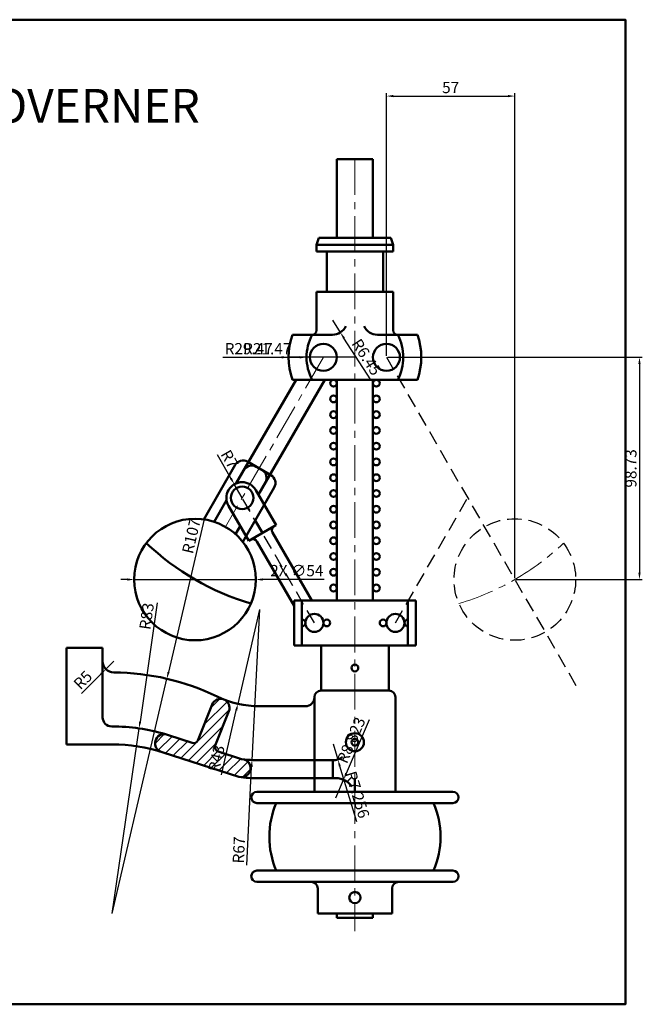
# Model space of a CAD drawing. Units: millimetres. Extents: x 98 to 674, y 38 to 476.
# Tile 7 of 7: x 398 to 674, y 38 to 476. Entities that reach past the tile are written whole.
import ezdxf

# ---------------------------------------------------------------- set-up
doc = ezdxf.new("R2010")
doc.units = ezdxf.units.MM
doc.header["$LTSCALE"] = 0.5
doc.linetypes.add('CENTER', pattern=[50.8, 31.75, -6.35, 6.35, -6.35])
doc.linetypes.add('DASHED', pattern=[19.05, 12.7, -6.35])
for name, color, linetype, lineweight in [('M-CNTR', 1, 'CENTER', 18), ('M-DIMS', 2, 'Continuous', 25), ('M-HATC', 8, 'Continuous', 18), ('M-OUTL', 7, 'Continuous', 50), ('M-PHAN', 6, 'DASHED', 25), ('M-TEXT', 3, 'Continuous', 25), ('M-TTLB', 7, 'Continuous', 50)]:
    doc.layers.add(name, color=color, linetype=linetype, lineweight=lineweight)
doc.styles.get("Standard").update_dxf_attribs({"font": 'arial.ttf'})
doc.dimstyles.new('ISO-25', dxfattribs={"dimtxt": 5, "dimasz": 3, "dimexe": 1.25, "dimexo": 0.625, "dimtad": 1, "dimtxsty": 'Standard', "dimcen": 2.5, "dimadec": 0, "dimazin": 0, "dimtfac": 1, "dimtmove": 0, "dimatfit": 3, "dimfxl": 1, "dimarcsym": 0})

# ---------------------------------------------------------------- blocks, each defined once
blk = doc.blocks.new('BALL')
blk.add_circle((27, 27), 27)
blk.add_arc((84, 125.73), 114, 226.398, 253.602)
blk = doc.blocks.new('*D69')
at = {"layer": 'Defpoints', "color": 0, "ltscale": 0.5, "transparency": 16777216}
for p in [(560.64, 325.69), (617.64, 226.96), (672.98, 226.96)]:
    blk.add_point(p, dxfattribs=at)
at = {"layer": 'M-DIMS', "color": 0, "lineweight": -2, "ltscale": 0.5, "transparency": 16777216}
for p, q in [((561.27, 325.69), (674.23, 325.69)), ((672.98, 322.69), (672.98, 229.96)), ((618.27, 226.96), (674.23, 226.96))]:
    blk.add_line(p, q, dxfattribs=at)
at = {"layer": 'M-DIMS', "color": 0, "ltscale": 0.5, "transparency": 16777216}
for points in [[(672.48, 322.69), (673.48, 322.69), (672.98, 325.69)], [(672.48, 229.96), (673.48, 229.96), (672.98, 226.96)]]:
    blk.add_solid(points, dxfattribs=at)
at = {"layer": 'M-DIMS', "color": 0, "ltscale": 0.5, "transparency": 16777216, "insert": (669.8, 276.32), "char_height": 5, "attachment_point": 5, "rotation": 90}
blk.add_mtext('98.73', dxfattribs=at)
blk = doc.blocks.new('*D70')
at = {"layer": 'Defpoints', "color": 0, "ltscale": 0.5, "transparency": 16777216}
for p in [(617.64, 441.69), (560.64, 325.69), (617.64, 226.96)]:
    blk.add_point(p, dxfattribs=at)
at = {"layer": 'M-DIMS', "color": 0, "lineweight": -2, "ltscale": 0.5, "transparency": 16777216}
for p, q in [((560.64, 326.31), (560.64, 442.94)), ((617.64, 227.58), (617.64, 442.94)), ((563.64, 441.69), (614.64, 441.69))]:
    blk.add_line(p, q, dxfattribs=at)
at = {"layer": 'M-DIMS', "color": 0, "ltscale": 0.5, "transparency": 16777216}
for points in [[(563.64, 442.19), (563.64, 441.19), (560.64, 441.69)], [(614.64, 442.19), (614.64, 441.19), (617.64, 441.69)]]:
    blk.add_solid(points, dxfattribs=at)
at = {"layer": 'M-DIMS', "color": 0, "ltscale": 0.5, "transparency": 16777216, "insert": (589.14, 444.85), "char_height": 5, "attachment_point": 5}
blk.add_mtext('57', dxfattribs=at)
blk = doc.blocks.new('*D75')
at = {"layer": 'Defpoints', "color": 0, "ltscale": 0.5, "transparency": 16777216}
for p in [(439.64, 190.68), (436.09, 187.16)]:
    blk.add_point(p, dxfattribs=at)
at = {"layer": 'M-DIMS', "color": 0, "lineweight": -2, "ltscale": 0.5, "transparency": 16777216}
for p, q in [((439.64, 190.68), (436.09, 187.16)), ((425.2, 176.34), (433.96, 185.04))]:
    blk.add_line(p, q, dxfattribs=at)
at = {"layer": 'M-DIMS', "color": 0, "ltscale": 0.5, "transparency": 16777216}
blk.add_solid([(433.61, 185.4), (434.32, 184.69), (436.09, 187.16)], dxfattribs=at)
at = {"layer": 'M-DIMS', "color": 0, "ltscale": 0.5, "transparency": 16777216, "insert": (426.29, 181.88), "char_height": 5, "attachment_point": 5, "rotation": 44.812}
blk.add_mtext('R5', dxfattribs=at)
blk = doc.blocks.new('*D79')
at = {"layer": 'Defpoints', "color": 0, "ltscale": 0.5, "transparency": 16777216}
for p in [(448.64, 226.96), (502.64, 226.96)]:
    blk.add_point(p, dxfattribs=at)
at = {"layer": 'M-DIMS', "color": 0, "lineweight": -2, "ltscale": 0.5, "transparency": 16777216}
for p, q in [((445.64, 226.96), (442.64, 226.96)), ((448.64, 226.96), (502.64, 226.96)), ((533.03, 226.96), (505.64, 226.96))]:
    blk.add_line(p, q, dxfattribs=at)
at = {"layer": 'M-DIMS', "color": 0, "ltscale": 0.5, "transparency": 16777216}
for points in [[(445.64, 227.46), (445.64, 226.46), (448.64, 226.96)], [(505.64, 227.46), (505.64, 226.46), (502.64, 226.96)]]:
    blk.add_solid(points, dxfattribs=at)
at = {"layer": 'M-DIMS', "color": 0, "ltscale": 0.5, "transparency": 16777216, "insert": (520.84, 230.28), "char_height": 5, "attachment_point": 5, "rotation": 0.0009}
blk.add_mtext('2X ∅54', dxfattribs=at)
blk = doc.blocks.new('*D80')
at = {"layer": 'Defpoints', "color": 0, "ltscale": 0.5, "transparency": 16777216}
for p in [(463.16, 182.89), (438.88, 78.69)]:
    blk.add_point(p, dxfattribs=at)
at = {"layer": 'M-DIMS', "color": 0, "lineweight": -2, "ltscale": 0.5, "transparency": 16777216}
for p, q in [((479.67, 253.74), (463.84, 185.82)), ((438.88, 78.69), (463.16, 182.89))]:
    blk.add_line(p, q, dxfattribs=at)
at = {"layer": 'M-DIMS', "color": 0, "ltscale": 0.5, "transparency": 16777216}
blk.add_solid([(463.35, 185.93), (464.33, 185.7), (463.16, 182.89)], dxfattribs=at)
at = {"layer": 'M-DIMS', "color": 0, "ltscale": 0.5, "transparency": 16777216, "insert": (474.63, 246.14), "char_height": 5, "attachment_point": 5, "rotation": 76.8836}
blk.add_mtext('R107', dxfattribs=at)
blk = doc.blocks.new('*D81')
at = {"layer": 'Defpoints', "color": 0, "ltscale": 0.5, "transparency": 16777216}
for p in [(450.8, 160.82), (438.88, 78.69)]:
    blk.add_point(p, dxfattribs=at)
at = {"layer": 'M-DIMS', "color": 0, "lineweight": -2, "ltscale": 0.5, "transparency": 16777216}
for p, q in [((458.9, 216.64), (451.23, 163.79)), ((438.88, 78.69), (450.8, 160.82))]:
    blk.add_line(p, q, dxfattribs=at)
at = {"layer": 'M-DIMS', "color": 0, "ltscale": 0.5, "transparency": 16777216}
blk.add_solid([(450.73, 163.87), (451.72, 163.72), (450.8, 160.82)], dxfattribs=at)
at = {"layer": 'M-DIMS', "color": 0, "ltscale": 0.5, "transparency": 16777216, "insert": (454.8, 210.57), "char_height": 5, "attachment_point": 5, "rotation": 81.7426}
blk.add_mtext('R83', dxfattribs=at)
blk = doc.blocks.new('*D82')
at = {"layer": 'Defpoints', "color": 0, "ltscale": 0.5, "transparency": 16777216}
for p in [(504.26, 213.69), (500.92, 146.77)]:
    blk.add_point(p, dxfattribs=at)
at = {"layer": 'M-DIMS', "color": 0, "lineweight": -2, "ltscale": 0.5, "transparency": 16777216}
for p, q in [((504.26, 213.69), (500.92, 146.77)), ((498.59, 100.03), (500.77, 143.77))]:
    blk.add_line(p, q, dxfattribs=at)
at = {"layer": 'M-DIMS', "color": 0, "ltscale": 0.5, "transparency": 16777216}
blk.add_solid([(500.27, 143.8), (501.27, 143.75), (500.92, 146.77)], dxfattribs=at)
at = {"layer": 'M-DIMS', "color": 0, "ltscale": 0.5, "transparency": 16777216, "insert": (495.74, 106.78), "char_height": 5, "attachment_point": 5, "rotation": 87.1418}
blk.add_mtext('R67', dxfattribs=at)
blk = doc.blocks.new('*D83')
at = {"layer": 'Defpoints', "color": 0, "ltscale": 0.5, "transparency": 16777216}
for p in [(504.26, 213.69), (494.65, 171.77)]:
    blk.add_point(p, dxfattribs=at)
at = {"layer": 'M-DIMS', "color": 0, "lineweight": -2, "ltscale": 0.5, "transparency": 16777216}
for p, q in [((504.26, 213.69), (494.65, 171.77)), ((487.4, 140.2), (493.97, 168.85))]:
    blk.add_line(p, q, dxfattribs=at)
at = {"layer": 'M-DIMS', "color": 0, "ltscale": 0.5, "transparency": 16777216}
blk.add_solid([(493.49, 168.96), (494.46, 168.74), (494.65, 171.77)], dxfattribs=at)
at = {"layer": 'M-DIMS', "color": 0, "ltscale": 0.5, "transparency": 16777216, "insert": (485.78, 147.34), "char_height": 5, "attachment_point": 5, "rotation": 77.0793}
blk.add_mtext('R43', dxfattribs=at)
blk = doc.blocks.new('*D84')
at = {"layer": 'Defpoints', "color": 0, "ltscale": 0.5, "transparency": 16777216}
for p in [(541.59, 138.06), (538.1, 129.96)]:
    blk.add_point(p, dxfattribs=at)
at = {"layer": 'M-DIMS', "color": 0, "lineweight": -2, "ltscale": 0.5, "transparency": 16777216}
for p, q in [((553.02, 164.61), (542.78, 140.82)), ((538.1, 129.96), (541.59, 138.06))]:
    blk.add_line(p, q, dxfattribs=at)
at = {"layer": 'M-DIMS', "color": 0, "ltscale": 0.5, "transparency": 16777216}
blk.add_solid([(542.32, 141.02), (543.24, 140.62), (541.59, 138.06)], dxfattribs=at)
at = {"layer": 'M-DIMS', "color": 0, "ltscale": 0.5, "transparency": 16777216, "insert": (545.57, 155.35), "char_height": 5, "attachment_point": 5, "rotation": 66.6993}
blk.add_mtext('R8.823', dxfattribs=at)
blk = doc.blocks.new('*D85')
at = {"layer": 'Defpoints', "color": 0, "ltscale": 0.5, "transparency": 16777216}
for p in [(536.94, 153.94), (539.05, 147)]:
    blk.add_point(p, dxfattribs=at)
at = {"layer": 'M-DIMS', "color": 0, "lineweight": -2, "ltscale": 0.5, "transparency": 16777216}
for p, q in [((536.94, 153.94), (539.05, 147)), ((547.43, 119.33), (539.92, 144.12))]:
    blk.add_line(p, q, dxfattribs=at)
at = {"layer": 'M-DIMS', "color": 0, "ltscale": 0.5, "transparency": 16777216}
blk.add_solid([(540.39, 144.27), (539.44, 143.98), (539.05, 147)], dxfattribs=at)
at = {"layer": 'M-DIMS', "color": 0, "ltscale": 0.5, "transparency": 16777216, "insert": (547.15, 131.22), "char_height": 5, "attachment_point": 5, "rotation": 286.8594}
blk.add_mtext('R7.256', dxfattribs=at)
blk = doc.blocks.new('*D86')
at = {"layer": 'Defpoints', "color": 0, "ltscale": 0.5, "transparency": 16777216}
for p in [(493.08, 269.28), (496.58, 263.22)]:
    blk.add_point(p, dxfattribs=at)
at = {"layer": 'M-DIMS', "color": 0, "lineweight": -2, "ltscale": 0.5, "transparency": 16777216}
for p, q in [((485.42, 282.54), (491.58, 271.88)), ((496.58, 263.22), (493.08, 269.28))]:
    blk.add_line(p, q, dxfattribs=at)
at = {"layer": 'M-DIMS', "color": 0, "ltscale": 0.5, "transparency": 16777216}
blk.add_solid([(492.01, 272.13), (491.14, 271.63), (493.08, 269.28)], dxfattribs=at)
at = {"layer": 'M-DIMS', "color": 0, "ltscale": 0.5, "transparency": 16777216, "insert": (490.45, 280.07), "char_height": 5, "attachment_point": 5, "rotation": 300.0011}
blk.add_mtext('R7', dxfattribs=at)
blk = doc.blocks.new('*D87')
at = {"layer": 'Defpoints', "color": 0, "ltscale": 0.5, "transparency": 16777216}
for p in [(517.17, 325.68), (546.64, 325.69)]:
    blk.add_point(p, dxfattribs=at)
at = {"layer": 'M-DIMS', "color": 0, "lineweight": -2, "ltscale": 0.5, "transparency": 16777216}
for p, q in [((488.03, 325.68), (514.17, 325.68)), ((546.64, 325.69), (517.17, 325.68))]:
    blk.add_line(p, q, dxfattribs=at)
at = {"layer": 'M-DIMS', "color": 0, "ltscale": 0.5, "transparency": 16777216}
blk.add_solid([(514.17, 326.18), (514.17, 325.18), (517.17, 325.68)], dxfattribs=at)
at = {"layer": 'M-DIMS', "color": 0, "ltscale": 0.5, "transparency": 16777216, "insert": (499.49, 328.86), "char_height": 5, "attachment_point": 5, "rotation": 0.0009}
blk.add_mtext('R29.47', dxfattribs=at)
blk = doc.blocks.new('*D88')
at = {"layer": 'Defpoints', "color": 0, "ltscale": 0.5, "transparency": 16777216}
for p in [(525.17, 325.68), (546.64, 325.69)]:
    blk.add_point(p, dxfattribs=at)
at = {"layer": 'M-DIMS', "color": 0, "lineweight": -2, "ltscale": 0.5, "transparency": 16777216}
for p, q in [((496.26, 325.68), (522.17, 325.68)), ((546.64, 325.69), (525.17, 325.68))]:
    blk.add_line(p, q, dxfattribs=at)
at = {"layer": 'M-DIMS', "color": 0, "ltscale": 0.5, "transparency": 16777216}
blk.add_solid([(522.17, 326.18), (522.17, 325.18), (525.17, 325.68)], dxfattribs=at)
at = {"layer": 'M-DIMS', "color": 0, "ltscale": 0.5, "transparency": 16777216, "insert": (507.72, 328.82), "char_height": 5, "attachment_point": 5, "rotation": 0.0013}
blk.add_mtext('R21.47', dxfattribs=at)
blk = doc.blocks.new('*D89')
at = {"layer": 'Defpoints', "color": 0, "ltscale": 0.5, "transparency": 16777216}
for p in [(536.65, 342.14), (540.15, 336.72)]:
    blk.add_point(p, dxfattribs=at)
at = {"layer": 'M-DIMS', "color": 0, "lineweight": -2, "ltscale": 0.5, "transparency": 16777216}
for p, q in [((536.65, 342.14), (540.15, 336.72)), ((553.77, 315.69), (541.78, 334.2))]:
    blk.add_line(p, q, dxfattribs=at)
at = {"layer": 'M-DIMS', "color": 0, "ltscale": 0.5, "transparency": 16777216}
blk.add_solid([(542.2, 334.48), (541.36, 333.93), (540.15, 336.72)], dxfattribs=at)
at = {"layer": 'M-DIMS', "color": 0, "ltscale": 0.5, "transparency": 16777216, "insert": (551.26, 325.41), "char_height": 5, "attachment_point": 5, "rotation": 302.9254}
blk.add_mtext('R6.45', dxfattribs=at)

msp = doc.modelspace()

# ---------------------------------------------------------------- hatches: boundary and pattern name
at = {"layer": 'M-HATC', "ltscale": 0.5}
h = msp.add_hatch(dxfattribs=at)
h.set_pattern_fill('ANSI31', color=256)
h.set_pattern_definition([(45, (694.353, 0), (-2.245064, 2.245064), [])])
h.paths.add_polyline_path([(476.9316, 155.5371, -0.39645231), (474.4505, 154.3725), (463.8044, 157.8537, 1), (460.1323, 150.6104, -0.00464805), (461.4658, 150.2028), (495.038, 139.3083, 1.17062936), (496.2913, 147.2309), (485.8775, 150.6361, -0.43220072), (484.6396, 153.2734), (490.6748, 168.5142, 1), (483.2367, 171.4596)])

# ---------------------------------------------------------------- linework, layer by layer
at = {"layer": 'M-CNTR'}
for p, q in [((546.6401, 413.6855), (546.6401, 70.7639)), ((532.6401, 325.6855), (489.1401, 250.3413))]:
    msp.add_line(p, q, dxfattribs=at)
msp.add_arc((560.6401, 325.6855), 114, 286.398028, 313.601972, dxfattribs=at)
at = {"layer": 'M-OUTL'}
for p, q in [((538.6401, 413.6855), (554.6401, 413.6855)), ((538.6401, 378.6855), (538.6401, 413.6855)), ((554.6401, 413.6855), (554.6401, 378.6855)), ((530.6401, 378.6855), (529.6401, 375.6855)), ((546.6401, 378.6855), (530.6401, 378.6855)), ((554.6401, 378.6855), (538.6401, 378.6855)), ((546.6401, 378.6855), (562.6401, 378.6855)), ((562.6401, 378.6855), (563.6401, 375.6855)), ((563.6401, 375.6855), (529.6401, 375.6855)), ((529.6401, 375.6855), (529.6401, 372.6855)), ((529.6401, 372.6855), (563.6401, 372.6855)), ((534.1401, 372.6855), (534.1401, 354.6855)), ((559.1401, 372.6855), (534.1401, 372.6855)), ((559.1401, 354.6855), (559.1401, 372.6855)), ((563.6401, 372.6855), (563.6401, 375.6855)), ((563.6401, 354.6855), (529.6401, 354.6855)), ((529.6401, 354.6855), (529.6401, 337.6855)), ((534.1401, 354.6855), (559.1401, 354.6855)), ((563.6401, 337.6855), (563.6401, 354.6855)), ((518.9176, 335.6855), (527.6401, 335.6855)), ((527.6401, 335.6855), (536.6401, 335.6855)), ((556.6274, 335.6855), (565.6401, 335.6855)), ((565.6401, 335.6855), (574.3625, 335.6855)), ((520.5157, 315.6855), (493.9783, 269.7214)), ((533.2174, 315.6855), (503.7933, 264.7214)), ((574.3625, 315.6855), (518.9176, 315.6855)), ((538.6401, 315.6855), (537.1401, 315.6855)), ((538.6401, 315.6855), (554.6401, 315.6855)), ((538.6401, 217.6855), (538.6401, 315.6855)), ((554.6401, 315.6855), (554.6401, 217.6855)), ((554.6401, 315.6855), (556.1401, 315.6855)), ((489.6482, 262.2214), (484.0939, 252.601)), ((495.7104, 250.7214), (493.6202, 247.101)), ((519.6401, 217.6855), (519.6401, 197.6855)), ((573.6401, 217.6855), (519.6401, 217.6855)), ((523.1401, 217.6855), (523.1401, 197.6855)), ((554.6401, 217.6855), (538.6401, 217.6855)), ((570.1401, 197.6855), (570.1401, 217.6855)), ((573.6401, 197.6855), (573.6401, 217.6855)), ((519.6401, 197.6855), (573.6401, 197.6855)), ((561.6401, 197.6855), (531.6401, 197.6855)), ((531.6401, 197.6855), (531.6401, 177.6855)), ((561.6401, 177.6855), (561.6401, 197.6855)), ((531.6401, 177.6855), (561.6401, 177.6855)), ((531.6401, 177.6855), (561.6401, 177.6855)), ((528.6401, 132.6855), (528.6401, 174.6855)), ((564.6401, 174.6855), (564.6401, 132.6855)), ((536.7953, 146.6855), (504.2599, 146.6855)), ((536.7953, 138.6855), (504.2599, 138.6855)), ((564.6401, 132.6855), (528.6401, 132.6855)), ((566.1401, 92.6855), (590.1401, 92.6855)), ((530.1401, 78.6855), (530.1401, 89.6855)), ((563.1401, 89.6855), (563.1401, 78.6855)), ((563.1401, 78.6855), (530.1401, 78.6855)), ((538.6401, 78.6855), (554.6401, 78.6855)), ((538.6401, 76.6855), (538.6401, 78.6855)), ((554.6401, 76.6855), (538.6401, 76.6855)), ((554.6401, 78.6855), (554.6401, 76.6855))]:
    msp.add_line(p, q, dxfattribs=at)
at = {"layer": 'M-OUTL', "ltscale": 0.7}
for p, q in [((493.4798, 277.8579), (479.5198, 253.6784)), ((509.6181, 273.1432), (498.9439, 279.322)), ((505.4391, 275.572), (502.841, 277.072)), ((496.8403, 243.6784), (510.8003, 267.8579)), ((502.6386, 266.7214), (511.6386, 251.1329)), ((490.5142, 259.7214), (499.5142, 244.1329)), ((499.0764, 258.8913), (499.7518, 257.7214)), ((510.7726, 250.6329), (499.5142, 244.1329)), ((502.3499, 253.2214), (505.5764, 247.6329)), ((510.7726, 250.6329), (511.6386, 251.1329))]:
    msp.add_line(p, q, dxfattribs=at)
at = {"layer": 'M-OUTL', "ltscale": 0.5}
for p, q in [((510.0405, 247.9009), (527.4854, 217.6855)), ((503.1123, 243.9009), (519.6401, 215.2739)), ((418.6401, 153.6855), (418.6401, 196.6855)), ((418.6401, 196.6855), (434.6401, 196.6855)), ((434.6401, 190.6829), (434.6401, 165.6855)), ((476.9316, 155.5371), (483.2367, 171.4596)), ((484.6396, 153.2734), (490.6748, 168.5142)), ((438.8764, 161.6855), (438.6401, 161.6855)), ((463.8044, 157.8537), (474.4505, 154.3725)), ((418.6401, 153.6855), (438.8764, 153.6855)), ((461.4658, 150.2028), (495.038, 139.3083)), ((485.8775, 150.6361), (496.2913, 147.2309)), ((536.7953, 146.6855), (536.7953, 138.6855)), ((546.6401, 132.6855), (546.6401, 138.6855))]:
    msp.add_line(p, q, dxfattribs=at)
at = {"layer": 'M-OUTL'}
msp.add_lwpolyline([(528.6401, 174.6855), (528.6401, 174.6855, -0.41421356), (524.6401, 170.6855), (504.2599, 170.6855, -0.11323701), (485.5167, 174.9855, 0.11151094), (439.606, 185.683, -0.41221797), (434.6401, 190.6829), (434.6401, 196.6855)], format="xyb", dxfattribs=at)
for points in [[(590.1401, 132.6855), (503.1401, 132.6855, 1), (503.1401, 127.6855), (590.1401, 127.6855, 1)], [(590.1401, 97.6855), (503.1401, 97.6855, 1), (503.1401, 92.6855), (590.1401, 92.6855, 1)]]:
    msp.add_lwpolyline(points, format="xyb", close=True, dxfattribs=at)
for centre, radius in [((532.6401, 325.6855), 6), ((560.6401, 325.6855), 6), ((537.1401, 314.1855), 1.5), ((556.1401, 314.1855), 1.5), ((537.1401, 307.1855), 1.5), ((556.1401, 307.1855), 1.5), ((537.1401, 300.1855), 1.5), ((556.1401, 300.1855), 1.5), ((537.1401, 293.1855), 1.5), ((556.1401, 293.1855), 1.5), ((537.1401, 286.1855), 1.5), ((556.1401, 286.1855), 1.5), ((537.1401, 279.1855), 1.5), ((556.1401, 279.1855), 1.5), ((537.1401, 272.1855), 1.5), ((556.1401, 272.1855), 1.5), ((537.1401, 265.1855), 1.5), ((556.1401, 265.1855), 1.5), ((537.1401, 258.1855), 1.5), ((556.1401, 258.1855), 1.5), ((537.1401, 251.1855), 1.5), ((556.1401, 251.1855), 1.5), ((537.1401, 244.1855), 1.5), ((556.1401, 244.1855), 1.5), ((537.1401, 237.1855), 1.5), ((556.1401, 237.1855), 1.5), ((537.1401, 230.1855), 1.5), ((556.1401, 230.1855), 1.5), ((537.1401, 223.1855), 1.5), ((556.1401, 223.1855), 1.5), ((528.6401, 207.6855), 4), ((564.6401, 207.6855), 4), ((534.1401, 207.6855), 1.5), ((559.1401, 207.6855), 1.5), ((546.6401, 154.6855), 4), ((546.6401, 154.6855), 1.5), ((546.6401, 85.6855), 2.5)]:
    msp.add_circle(centre, radius, dxfattribs=at)
at = {"layer": 'M-OUTL', "ltscale": 0.7}
msp.add_circle((496.5764, 263.2214), 5, dxfattribs=at)
at = {"layer": 'M-OUTL', "ltscale": 0.5}
msp.add_circle((546.6401, 187.6855), 1.5, dxfattribs=at)
at = {"layer": 'M-OUTL'}
for centre, radius, start, end in [((527.6401, 337.6855), 2, 270, 0), ((536.6464, 342.1355), 6.4501, 269.943606, 335.909896), ((556.6337, 342.1355), 6.4501, 204.090104, 270.056394), ((565.6401, 337.6855), 2, 180, 270), ((546.6401, 325.6855), 29.4709, 160.164693, 199.835307), ((546.6401, 325.6855), 21.4709, 152.241459, 207.758541), ((546.6401, 325.6855), 21.4709, 332.241459, 27.758541), ((546.6401, 325.6855), 29.4709, 340.164693, 19.835307), ((523.1401, 207.6855), 1.5, 270, 90), ((570.1401, 207.6855), 1.5, 90, 270), ((531.6401, 174.6855), 3, 90, 180), ((561.6401, 174.6855), 3, 0, 90), ((438.8764, 78.6855), 83, 73.484775, 90), ((438.8764, 78.6855), 75, 72.470867, 90), ((504.2599, 213.6855), 67, 264.284271, 270), ((504.2599, 213.6855), 75, 263.900929, 270), ((546.6401, 112.6855), 38, 156.750437, 203.249563), ((546.6401, 112.6855), 38, 336.750437, 23.249563), ((527.1401, 89.6855), 3, 0, 90), ((566.1401, 89.6855), 3, 90, 180)]:
    msp.add_arc(centre, radius, start, end, dxfattribs=at)
at = {"layer": 'M-OUTL', "ltscale": 0.7}
for centre, radius, start, end in [((496.9439, 275.8579), 4, 60, 150), ((500.841, 273.6079), 4, 60, 150), ((503.4391, 272.1079), 4, 330, 60), ((507.3362, 269.8579), 4, 330, 60), ((496.5764, 263.2214), 7, 30, 210)]:
    msp.add_arc(centre, radius, start, end, dxfattribs=at)
at = {"layer": 'M-OUTL', "ltscale": 0.5}
for centre, radius, start, end in [((511.7726, 248.9009), 2, 120, 210), ((501.3803, 242.9009), 2, 30, 120), ((486.9557, 169.9869), 4, 338.396932, 158.396932), ((438.6401, 165.6855), 4, 180, 270), ((461.9683, 154.232), 4.0605, 63.116651, 243.116651), ((475.0721, 156.2735), 2, 251.893074, 338.396932), ((486.4991, 152.537), 2, 158.396932, 251.893074), ((496.2913, 143.1705), 4.0605, 252.021289, 90), ((536.9417, 153.9397), 7.2557, 268.843493, 304.869517), ((538.0998, 129.959), 8.8234, 34.895768, 98.502029)]:
    msp.add_arc(centre, radius, start, end, dxfattribs=at)
at = {"layer": 'M-PHAN'}
for p, q in [((560.6401, 325.6855), (644.9803, 179.6039)), ((528.6401, 207.6855), (496.5764, 263.2214)), ((564.6401, 207.6855), (596.7037, 263.2214))]:
    msp.add_line(p, q, dxfattribs=at)
msp.add_circle((617.6401, 226.9586), 27, dxfattribs=at)
at = {"layer": 'M-TTLB', "ltscale": 0.5}
msp.add_lwpolyline([(98.2162, 475.6271), (666.7064, 475.6271), (666.7064, 38.2873), (98.2162, 38.2873)], close=True, dxfattribs=at)

# ---------------------------------------------------------------- block references
at = {"layer": 'M-OUTL'}
msp.add_blockref('BALL', (448.6401, 199.959), dxfattribs=at)

# ---------------------------------------------------------------- texts
at = {"layer": 'M-TEXT', "ltscale": 0.5, "insert": (319.1609, 444.8561), "char_height": 15, "attachment_point": 1}
msp.add_mtext_dynamic_manual_height_columns('BALL GOVERNER', width=187.408111, gutter_width=12.5, heights=[0], dxfattribs=at)

# ---------------------------------------------------------------- dimensions: what is measured, and where the dimension line sits
at = {"layer": 'M-DIMS', "ltscale": 0.5}
dim = msp.add_linear_dim(base=(617.6401, 441.6855), p1=(560.6401, 325.6855), p2=(617.6401, 226.9586), dimstyle='ISO-25', override={"dimdec": 0, "dimlfac": 1, "dimrnd": 0, "dimzin": 0, "dimdsep": 46, "dimlunit": 2}, dxfattribs=at)
dim.commit()
dim.dimension.update_dxf_attribs({"geometry": '*D70', "text_midpoint": (589.1401, 444.8531)})
for center, mpoint, override, picture, middle in [((536.6464, 342.1355), (540.1523, 336.7215), {"dimdec": 2, "dimlfac": 1, "dimrnd": 0, "dimzin": 0, "dimdsep": 46, "dimlunit": 2}, '*D89', (551.2611, 325.4131)), ((546.6401, 325.6855), (525.1692, 325.685), {"dimdec": 2, "dimlfac": 1, "dimrnd": 0, "dimzin": 0, "dimdsep": 46, "dimlunit": 2}, '*D88', (507.7153, 328.8198)), ((496.5764, 263.2214), (493.0763, 269.2835), {"dimdec": 0, "dimlfac": 1, "dimrnd": 0, "dimzin": 0, "dimdsep": 46, "dimlunit": 2}, '*D86', (490.4542, 280.0746)), ((439.6401, 190.6829), (436.093, 187.159), {"dimdec": 0, "dimlfac": 1, "dimrnd": 0, "dimzin": 0, "dimdsep": 46, "dimlunit": 2}, '*D75', (426.2873, 181.8825)), ((538.0998, 129.959), (541.5899, 138.0628), {"dimdec": 3, "dimlfac": 1, "dimrnd": 0, "dimzin": 0, "dimdsep": 46, "dimlunit": 2}, '*D84', (545.5736, 155.3508)), ((536.9417, 153.9397), (539.046, 146.9959), {"dimdec": 3, "dimlfac": 1, "dimrnd": 0, "dimzin": 0, "dimdsep": 46, "dimlunit": 2}, '*D85', (547.1488, 131.2155))]:
    dim = msp.add_radius_dim(center=center, mpoint=mpoint, dimstyle='ISO-25', override=override, dxfattribs=at)
    dim.commit()
    dim.dimension.update_dxf_attribs({"geometry": picture, "text_midpoint": middle})
for center, mpoint, override, picture, middle in [((546.6401, 325.6855), (517.1692, 325.685), {"dimdec": 2, "dimlfac": 1, "dimrnd": 0, "dimzin": 0, "dimdsep": 46, "dimlunit": 2}, '*D87', (499.4866, 325.6847)), ((438.8764, 78.6855), (463.158, 182.894), {"dimdec": 0, "dimlfac": 1, "dimrnd": 0, "dimzin": 0, "dimdsep": 46, "dimlunit": 2}, '*D80', (477.7269, 245.419)), ((438.8764, 78.6855), (450.797, 160.825), {"dimdec": 0, "dimlfac": 1, "dimrnd": 0, "dimzin": 0, "dimdsep": 46, "dimlunit": 2}, '*D81', (457.9493, 210.1087)), ((504.2599, 213.6855), (494.6451, 171.7742), {"dimdec": 0, "dimlfac": 1, "dimrnd": 0, "dimzin": 0, "dimdsep": 46, "dimlunit": 2}, '*D83', (488.8761, 146.6275)), ((504.2599, 213.6855), (500.919, 146.7688), {"dimdec": 0, "dimlfac": 1, "dimrnd": 0, "dimzin": 0, "dimdsep": 46, "dimlunit": 2}, '*D82', (498.9144, 106.6188))]:
    dim = msp.add_radius_dim(center=center, mpoint=mpoint, dimstyle='ISO-25', override=override, dxfattribs=at)
    dim.commit()
    dim.dimension.update_dxf_attribs({"geometry": picture, "text_midpoint": middle, "dimtype": 164})
dim = msp.add_linear_dim(base=(672.9803, 226.9586), p1=(560.6401, 325.6855), p2=(617.6401, 226.9586), angle=90, dimstyle='ISO-25', override={"dimdec": 2, "dimlfac": 1, "dimrnd": 0, "dimzin": 0, "dimdsep": 46, "dimlunit": 2}, dxfattribs=at)
dim.commit()
dim.dimension.update_dxf_attribs({"geometry": '*D69', "text_midpoint": (669.8008, 276.322)})
dim = msp.add_diameter_dim_2p(p1=(448.6401, 226.9582), p2=(502.6401, 226.959), text='2X <>', dimstyle='ISO-25', override={"dimdec": 0, "dimlfac": 1, "dimrnd": 0, "dimzin": 0, "dimdsep": 46, "dimlunit": 2}, dxfattribs=at)
dim.commit()
dim.dimension.update_dxf_attribs({"geometry": '*D79', "text_midpoint": (520.8374, 226.9593)})

doc.saveas('drawing.dxf')
